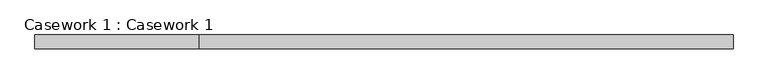
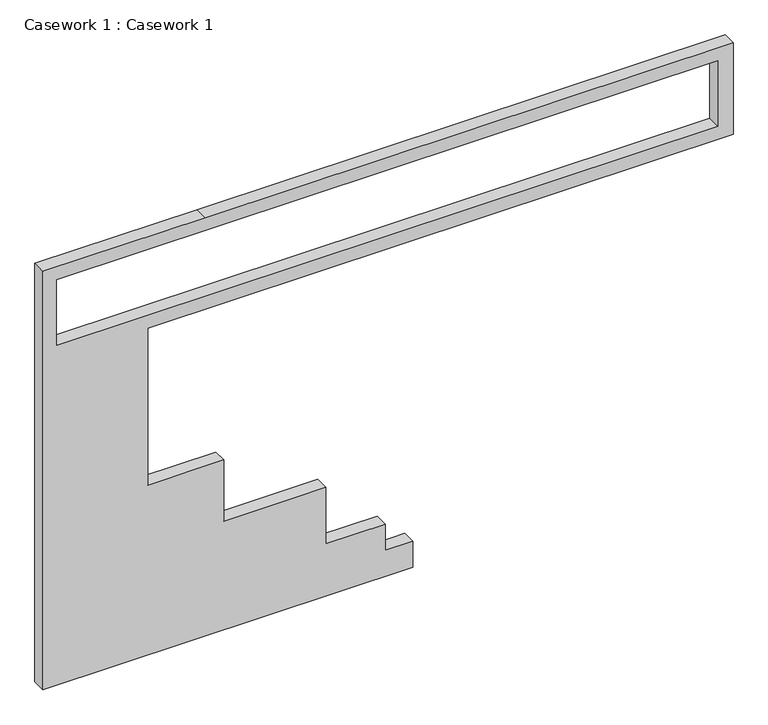
"""IFC4 building model written with IfcOpenShell, lengths in millimetres: furniture geometry, Casework 1 : Casework 1."""

from ifc_helpers import new_model, si_unit, frame, origin, place, context, project, spatial, polyline, outline, extrude, source, transform, mapped, element, save


def casework_1_casework_1_0d475414(model_context):
    return source(origin(), model_context, "Body", "SweptSolid", [
        extrude(outline(polyline([(0.0, 19013.3136801), (0.0, 23090.0136801), (304.8, 23090.0136801), (304.8, 22785.2136801), (609.6, 22785.2136801), (609.6, 22131.1636801), (1270.0, 22131.1636801), (1270.0, 21007.2136801), (1981.2, 21007.2136801), (1981.2, 20169.0136801), (3810.0, 20169.0136801), (3810.0, 26620.6136801), (4876.8, 26620.6136801), (4876.8, 20804.0136801), (4876.8, 19013.3136801), (0.0, 19013.3136801)]), holes=[polyline([(4724.4, 26452.1349515), (3962.4, 26452.1349515), (3962.4, 19165.7136801), (4724.4, 19165.7136801), (4724.4, 26452.1349515)])]), frame((0.0, 3125.1752787, 0.0), z_axis=(0.0, 1.0, 0.0), x_axis=(0.0, 0.0, 1.0)), (0.0, 0.0, 1.0), 152.4),
    ])


if __name__ == "__main__":
    model = new_model("IFC4")
    model_context = context("Model", 3, world=origin())
    ifc_project = project(units=[si_unit("LENGTHUNIT", "METRE", prefix="MILLI")], contexts=[model_context])
    site = spatial("IfcSite", under=ifc_project)
    building = spatial("IfcBuilding", under=site)
    placement = place(None, origin())
    casework_1_casework_1_shape = casework_1_casework_1_0d475414(model_context)
    element("IfcFurniture", 1, ObjectType="Casework 1 : Casework 1", at=placement, inside=building, context=model_context, shape_type="MappedRepresentation", body=[
        mapped(casework_1_casework_1_shape, transform((0.0, 0.0, 0.0), x_axis=(1.0, 0.0, 0.0), y_axis=(0.0, 1.0, 0.0), z_axis=(0.0, 0.0, 1.0))),
    ])
    save(model, "model.ifc")

# Revit data of these elements
# Element 1 (IfcFurniture, "Casework 1 : Casework 1")
#   Materials on its faces: "Birch"
# Materials
#   "Birch": class "Wood", colour RGB 224 178 126, transparency 0, Description = "Betula Alleghaniensis", Cost = 0
